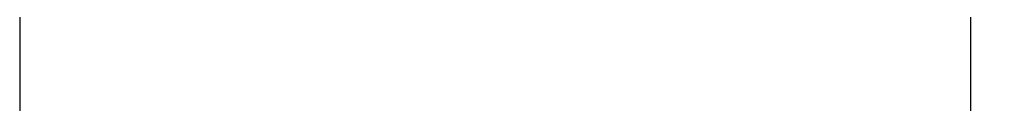
# Model space of a CAD drawing. Units: inches. Extents: x 2091 to 2899, y 967 to 2217.
# Tile 5 of 256: x 2212 to 2312, y 1081 to 1089. Entities that reach past the tile are written whole.
import ezdxf

# ---------------------------------------------------------------- set-up
doc = ezdxf.new("R2010")
doc.units = ezdxf.units.IN
doc.layers.add('A-ANNO-DIMS', color=2, linetype='Continuous', lineweight=18)
doc.styles.get("Standard").update_dxf_attribs({"font": 'arial.ttf'})
doc.dimstyles.new('ISO-25', dxfattribs={"dimtxt": 4, "dimasz": 4, "dimexe": 1.25, "dimexo": 0.625, "dimtad": 1, "dimdec": 0, "dimlunit": 3, "dimtxsty": 'Standard', "dimcen": 2.5, "dimadec": 0, "dimazin": 0, "dimtfac": 1, "dimtdec": 0, "dimtmove": 0, "dimatfit": 3, "dimfxl": 1, "dimarcsym": 0})

# ---------------------------------------------------------------- blocks, each defined once
blk = doc.blocks.new('*D71')
at = {"layer": 'A-ANNO-DIMS', "color": 0, "lineweight": -2, "transparency": 16777216}
for p, q in [((2212.144, 1351.294), (2212.144, 969.464)), ((2452.144, 1351.294), (2452.144, 969.464)), ((2216.144, 970.714), (2448.144, 970.714))]:
    blk.add_line(p, q, dxfattribs=at)
at = {"layer": 'A-ANNO-DIMS', "color": 0, "transparency": 16777216}
for points in [[(2216.144, 971.381), (2216.144, 970.048), (2212.144, 970.714)], [(2448.144, 971.381), (2448.144, 970.048), (2452.144, 970.714)]]:
    blk.add_solid(points, dxfattribs=at)
at = {"layer": 'Defpoints', "color": 0, "transparency": 16777216}
for p in [(2212.144, 1351.919), (2452.144, 1351.919), (2452.144, 970.714)]:
    blk.add_point(p, dxfattribs=at)
at = {"layer": 'A-ANNO-DIMS', "color": 0, "transparency": 16777216, "insert": (2332.144, 973.382), "char_height": 4, "attachment_point": 5}
blk.add_mtext('20\'-0"', dxfattribs=at)
blk = doc.blocks.new('*D75')
at = {"layer": 'A-ANNO-DIMS', "color": 0, "lineweight": -2, "transparency": 16777216}
for p, q in [((2212.144, 1274.794), (2212.144, 969.464)), ((2308.144, 1274.794), (2308.144, 969.464)), ((2216.144, 970.714), (2304.144, 970.714))]:
    blk.add_line(p, q, dxfattribs=at)
at = {"layer": 'A-ANNO-DIMS', "color": 0, "transparency": 16777216}
for points in [[(2216.144, 971.381), (2216.144, 970.048), (2212.144, 970.714)], [(2304.144, 971.381), (2304.144, 970.048), (2308.144, 970.714)]]:
    blk.add_solid(points, dxfattribs=at)
at = {"layer": 'Defpoints', "color": 0, "transparency": 16777216}
for p in [(2212.144, 1275.419), (2308.144, 1275.419), (2308.144, 970.714)]:
    blk.add_point(p, dxfattribs=at)
at = {"layer": 'A-ANNO-DIMS', "color": 0, "transparency": 16777216, "insert": (2260.144, 973.382), "char_height": 4, "attachment_point": 5}
blk.add_mtext('8\'-0"', dxfattribs=at)

msp = doc.modelspace()

# ---------------------------------------------------------------- dimensions: what is measured, and where the dimension line sits
at = {"layer": 'A-ANNO-DIMS'}
for base, p1, p2, picture, middle in [((2452.144, 970.714), (2212.144, 1351.919), (2452.144, 1351.919), '*D71', (2332.144, 973.382)), ((2308.144, 970.714), (2212.144, 1275.419), (2308.144, 1275.419), '*D75', (2260.144, 973.382))]:
    dim = msp.add_linear_dim(base=base, p1=p1, p2=p2, dimstyle='ISO-25', override={"dimdec": 1, "dimlfac": 1, "dimrnd": 0, "dimzin": 1, "dimdsep": 46, "dimlunit": 4, "dimfrac": 2}, dxfattribs=at)
    dim.commit()
    dim.dimension.update_dxf_attribs({"geometry": picture, "text_midpoint": middle})

doc.saveas('drawing.dxf')
